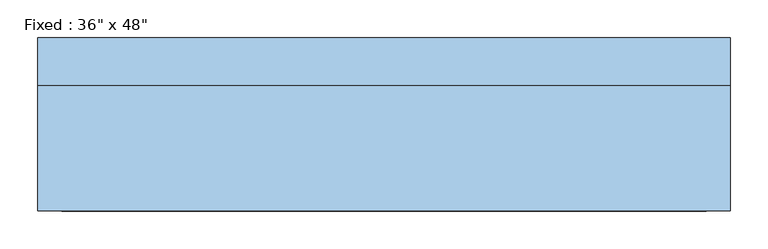
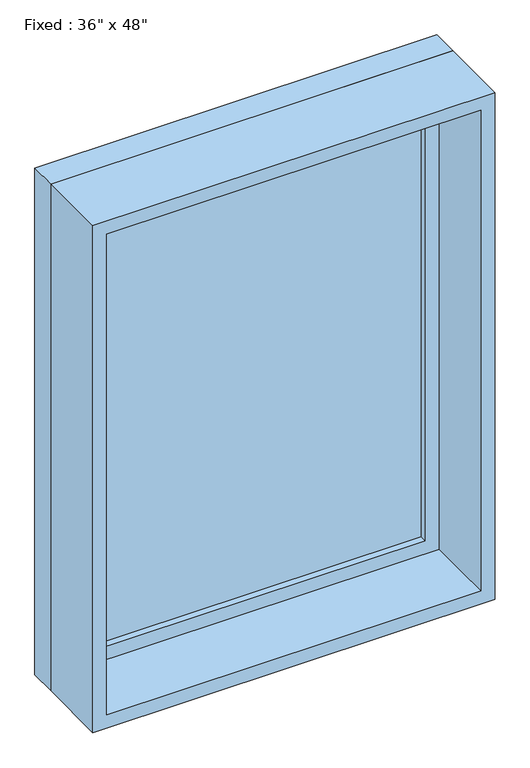
"""IFC4 building model written with IfcOpenShell, lengths in millimetres: window geometry."""

from ifc_helpers import new_model, si_unit, frame, origin, place, context, project, spatial, polyline, outline, extrude, source, transform, mapped, element, save


def window_c1f32544(model_context):
    return source(origin(), model_context, "Body", "SweptSolid", [
        extrude(outline(polyline([(355.6, 66.675), (-431.8, 66.675), (-431.8, 79.375), (355.6, 79.375), (355.6, 66.675)])), frame((0.0, 0.0, 977.9), z_axis=(0.0, 0.0, 1.0), x_axis=(1.0, 0.0, 0.0)), (0.0, 0.0, 1.0), 1092.2),
        extrude(outline(polyline([(2114.55, -476.25), (933.45, -476.25), (933.45, 400.05), (2114.55, 400.05), (2114.55, -476.25)]), holes=[polyline([(2070.1, -431.8), (2070.1, 355.6), (977.9, 355.6), (977.9, -431.8), (2070.1, -431.8)])]), frame((0.0, 50.8, 0.0), z_axis=(0.0, 1.0, 0.0), x_axis=(0.0, 0.0, 1.0)), (0.0, 0.0, 1.0), 44.45),
        extrude(outline(polyline([(2133.6, -495.3), (914.4, -495.3), (914.4, 419.1), (2133.6, 419.1), (2133.6, -495.3)]), holes=[polyline([(2101.85, -463.55), (2101.85, 387.35), (946.15, 387.35), (946.15, -463.55), (2101.85, -463.55)])]), frame((0.0, -114.3, 0.0), z_axis=(0.0, 1.0, 0.0), x_axis=(0.0, 0.0, 1.0)), (0.0, 0.0, 1.0), 165.1),
        extrude(outline(polyline([(2133.6, 419.1), (2133.6, -495.3), (914.4, -495.3), (914.4, 419.1), (2133.6, 419.1)]), holes=[polyline([(2114.55, 400.05), (933.45, 400.05), (933.45, -476.25), (2114.55, -476.25), (2114.55, 400.05)])]), frame((0.0, 50.8, 0.0), z_axis=(0.0, 1.0, 0.0), x_axis=(0.0, 0.0, 1.0)), (0.0, 0.0, 1.0), 63.5),
    ])


if __name__ == "__main__":
    model = new_model("IFC4")
    model_context = context("Model", 3, world=origin())
    ifc_project = project(units=[si_unit("LENGTHUNIT", "METRE", prefix="MILLI")], contexts=[model_context])
    site = spatial("IfcSite", under=ifc_project)
    building = spatial("IfcBuilding", under=site)
    placement = place(None, origin())
    window_shape = window_c1f32544(model_context)
    element("IfcWindow", 1, ObjectType="Fixed : 36\" x 48\"", at=placement, inside=building, context=model_context, shape_type="MappedRepresentation", body=[
        mapped(window_shape, transform((0.0, 0.0, 0.0), x_axis=(1.0, 0.0, 0.0), y_axis=(0.0, 1.0, 0.0), z_axis=(0.0, 0.0, 1.0))),
    ])
    save(model, "model.ifc")

# Revit data of these elements
# Type "Fixed : 36\" x 48\""
#   Type Mark = "9"
#   Construction Type Id = "GSP4R"
#   Assembly Code = "B2020100"
#   Analytic Construction = "1/8 in Pilkington single glazing"
#   Visual Light Transmittance = 0.9
#   Solar Heat Gain Coefficient = 0.78
#   Heat Transfer Coefficient (U) = 0.6496 BTU/(h·ft²·°F)
#   Height = 4' - 0"
#   Default Sill Height = 3' - 0"
#   Width = 3' - 0"
#   Window Inset = 0' - 0 3/4"
#   Define Thermal Properties by = 1
#   Wall Closure = 3
#   Glass Pane Material = Glass
#   Sash Material = Sash
# Element 1 (IfcWindow, "Fixed : 36\" x 48\"")
#   Materials on its faces: "Sash", "Glass"
# Materials
#   "Glass": class "Glass", colour RGB 0 128 192, transparency 0.75, Description = "Soda Lime Glass", Cost = 0
#   "Sash": class "Wood", colour RGB 224 178 126, transparency 0
